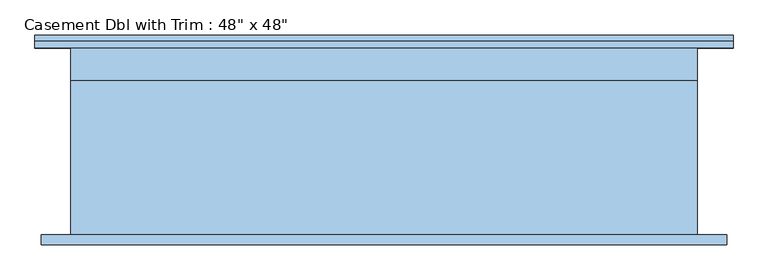
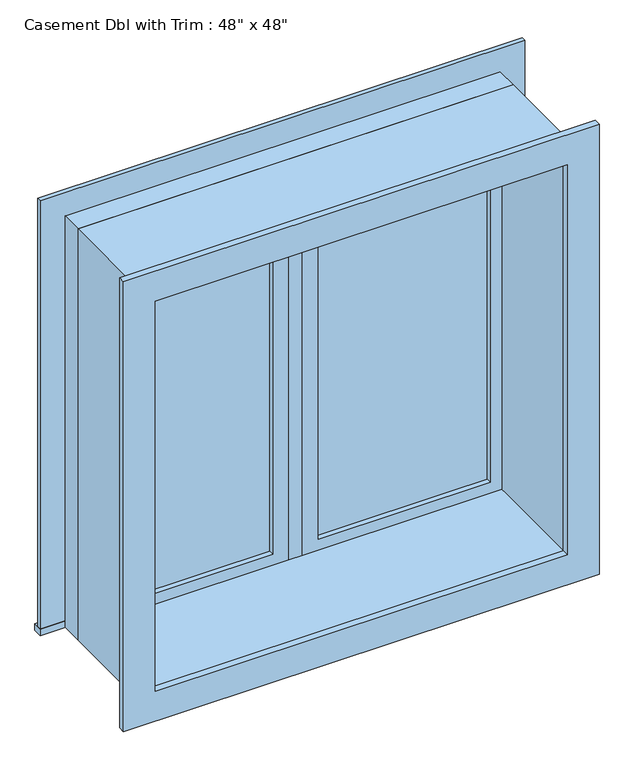
"""IFC4 building model written with IfcOpenShell, lengths in millimetres: window geometry."""

from ifc_helpers import new_model, si_unit, frame, origin, place, context, project, spatial, polyline, outline, extrude, source, transform, mapped, element, save


def window_6544a982(model_context):
    return source(origin(), model_context, "Body", "SweptSolid", [
        extrude(outline(polyline([(63.5, 165.9250007), (546.1, 165.9250007), (546.1, 153.2250007), (63.5, 153.2250007), (63.5, 165.9250007)])), frame((0.0, 0.0, 977.9), z_axis=(0.0, 0.0, 1.0), x_axis=(1.0, 0.0, 0.0)), (0.0, 0.0, 1.0), 1092.2),
        extrude(outline(polyline([(2114.55, 19.05), (933.45, 19.05), (933.45, 590.55), (2114.55, 590.55), (2114.55, 19.05)]), holes=[polyline([(2070.1, 63.5), (2070.1, 546.1), (977.9, 546.1), (977.9, 63.5), (2070.1, 63.5)])]), frame((0.0, 137.3500007, 0.0), z_axis=(0.0, 1.0, 0.0), x_axis=(0.0, 0.0, 1.0)), (0.0, 0.0, 1.0), 44.45),
        extrude(outline(polyline([(19.05, 137.3500007), (-19.05, 137.3500007), (-19.05, 200.8500007), (19.05, 200.8500007), (19.05, 137.3500007)])), frame((0.0, 0.0, 933.45), z_axis=(0.0, 0.0, 1.0), x_axis=(1.0, 0.0, 0.0)), (0.0, 0.0, 1.0), 1181.1),
        extrude(outline(polyline([(-679.45, 226.2500007), (679.45, 226.2500007), (679.45, 200.8500007), (-679.45, 200.8500007), (-679.45, 226.2500007)])), frame((0.0, 0.0, 914.4), z_axis=(0.0, 0.0, 1.0), x_axis=(1.0, 0.0, 0.0)), (0.0, 0.0, 1.0), 19.05),
        extrude(outline(polyline([(2114.55, -590.55), (2114.55, 590.55), (933.45, 590.55), (933.45, 679.45), (2203.45, 679.45), (2203.45, -679.45), (933.45, -679.45), (933.45, -590.55), (2114.55, -590.55)])), frame((0.0, 200.8500007, 0.0), z_axis=(0.0, 1.0, 0.0), x_axis=(0.0, 0.0, 1.0)), (0.0, 0.0, 1.0), 12.7),
        extrude(outline(polyline([(2190.75, 666.75), (2190.75, -666.75), (857.25, -666.75), (857.25, 666.75), (2190.75, 666.75)]), holes=[polyline([(2101.85, 577.85), (946.15, 577.85), (946.15, -577.85), (2101.85, -577.85), (2101.85, 577.85)])]), frame((0.0, -181.8000007, 0.0), z_axis=(0.0, 1.0, 0.0), x_axis=(0.0, 0.0, 1.0)), (0.0, 0.0, 1.0), 19.05),
        extrude(outline(polyline([(-63.5, 153.2250007), (-546.1, 153.2250007), (-546.1, 165.9250007), (-63.5, 165.9250007), (-63.5, 153.2250007)])), frame((0.0, 0.0, 977.9), z_axis=(0.0, 0.0, 1.0), x_axis=(1.0, 0.0, 0.0)), (0.0, 0.0, 1.0), 1092.2),
        extrude(outline(polyline([(2114.55, -590.55), (933.45, -590.55), (933.45, -19.05), (2114.55, -19.05), (2114.55, -590.55)]), holes=[polyline([(2070.1, -546.1), (2070.1, -63.5), (977.9, -63.5), (977.9, -546.1), (2070.1, -546.1)])]), frame((0.0, 137.3500007, 0.0), z_axis=(0.0, 1.0, 0.0), x_axis=(0.0, 0.0, 1.0)), (0.0, 0.0, 1.0), 44.45),
        extrude(outline(polyline([(2133.6, -609.6), (914.4, -609.6), (914.4, 609.6), (2133.6, 609.6), (2133.6, -609.6)]), holes=[polyline([(2101.85, -577.85), (2101.85, 577.85), (946.15, 577.85), (946.15, -577.85), (2101.85, -577.85)])]), frame((0.0, -162.7500007, 0.0), z_axis=(0.0, 1.0, 0.0), x_axis=(0.0, 0.0, 1.0)), (0.0, 0.0, 1.0), 300.1000013),
        extrude(outline(polyline([(2133.6, 609.6), (2133.6, -609.6), (914.4, -609.6), (914.4, 609.6), (2133.6, 609.6)]), holes=[polyline([(2114.55, 590.55), (933.45, 590.55), (933.45, -590.55), (2114.55, -590.55), (2114.55, 590.55)])]), frame((0.0, 137.3500007, 0.0), z_axis=(0.0, 1.0, 0.0), x_axis=(0.0, 0.0, 1.0)), (0.0, 0.0, 1.0), 63.5),
    ])


if __name__ == "__main__":
    model = new_model("IFC4")
    model_context = context("Model", 3, world=origin())
    ifc_project = project(units=[si_unit("LENGTHUNIT", "METRE", prefix="MILLI")], contexts=[model_context])
    site = spatial("IfcSite", under=ifc_project)
    building = spatial("IfcBuilding", under=site)
    placement = place(None, origin())
    window_shape = window_6544a982(model_context)
    element("IfcWindow", 1, ObjectType="Casement Dbl with Trim : 48\" x 48\"", at=placement, inside=building, context=model_context, shape_type="MappedRepresentation", body=[
        mapped(window_shape, transform((0.0, 0.0, 0.0), x_axis=(1.0, 0.0, 0.0), y_axis=(0.0, 1.0, 0.0), z_axis=(0.0, 0.0, 1.0))),
    ])
    save(model, "model.ifc")

# Revit data of these elements
# Type "Casement Dbl with Trim : 48\" x 48\""
#   Type Mark = "13"
#   Construction Type Id = "GSP4R"
#   Assembly Code = "B2020100"
#   Analytic Construction = "1/8 in Pilkington single glazing"
#   Visual Light Transmittance = 0.9
#   Solar Heat Gain Coefficient = 0.78
#   Heat Transfer Coefficient (U) = 0.6496 BTU/(h·ft²·°F)
#   Height = 4' - 0"
#   Default Sill Height = 3' - 0"
#   Trim Projection - Ext. = 0' - 0 1/2"
#   Trim Projection - Int. = 0' - 0 3/4"
#   Trim Width - Exterior = 0' - 3 1/2"
#   Trim Width - Interior = 0' - 3 1/2"
#   Width = 4' - 0"
#   Window Inset = 0' - 0 3/4"
#   Define Thermal Properties by = 1
#   Glass Pane Material = Glass
#   Sash Material = Sash
#   Trim Exterior Material = Trim
#   Trim Interior Material = Trim
#   Wall Closure = (empty or 0)
# Element 1 (IfcWindow, "Casement Dbl with Trim : 48\" x 48\"")
#   Materials on its faces: "Sash", "Trim", "Glass"
# Materials
#   "Glass": class "Glass", colour RGB 0 128 192, transparency 0.75, Description = "Soda Lime Glass", Cost = 0
#   "Sash": class "Wood", colour RGB 224 178 126, transparency 0
#   "Trim": class "Wood", colour RGB 224 178 126, transparency 0
